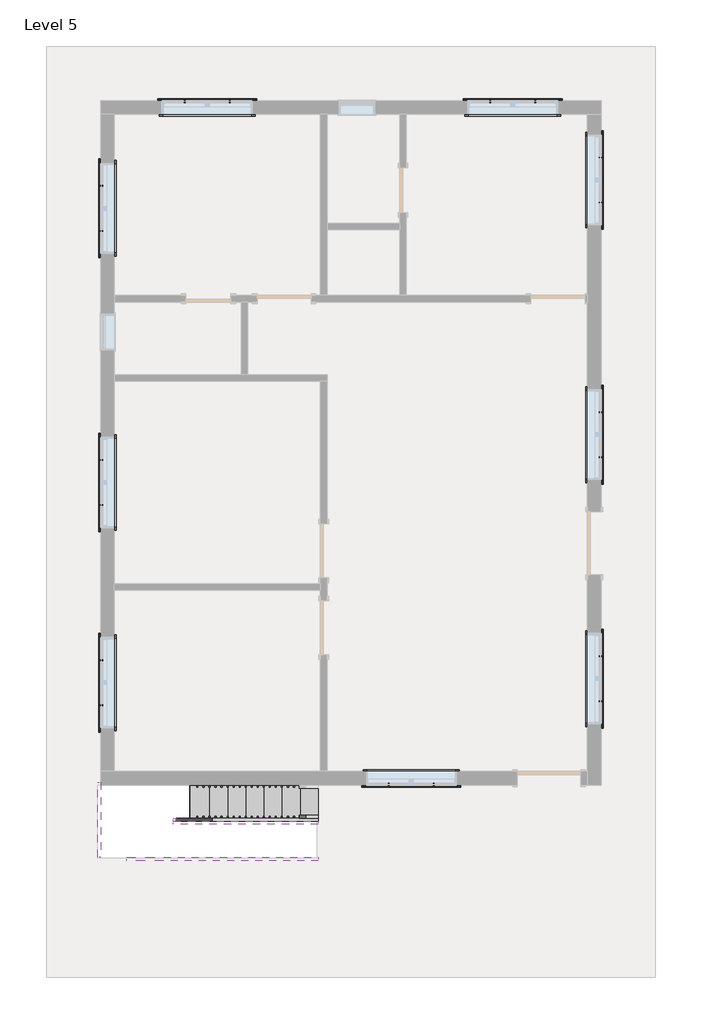
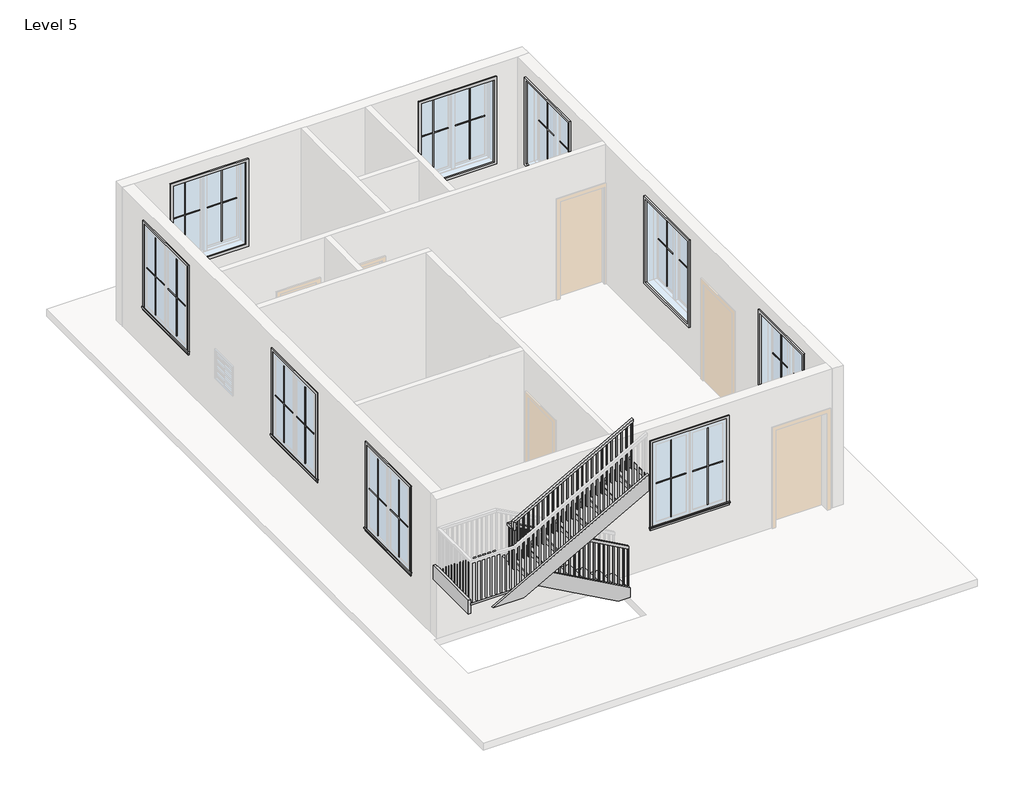
# One storey, part 3 of 3: 36 proxies, 6 members, 1 railing, 1 stair flight.
"""IFC4 building model written with IfcOpenShell, lengths in millimetres."""

from ifc_helpers import new_model, si_unit, frame, origin, place, context, project, spatial, polyline, outline, extrude, faceted_brep, transform, mapped, element, save
from components import muntin_pattern_2x2_muntin_pattern_2x2_f6a80940, muntin_pattern_2x2_muntin_pattern_2x2_09b00a1c, trim_window_exterior_flat_with_sill_698ed857, trim_window_interior_flat_picture_frame_92551a5e, stair_flight_d84c00c9

model = new_model("IFC4")

# Units and contexts
model_context = context("Model", 3, world=origin())
ifc_project = project(units=[si_unit("LENGTHUNIT", "METRE", prefix="MILLI")], contexts=[model_context])

# Site, building, storey
site = spatial("IfcSite", under=ifc_project)
building = spatial("IfcBuilding", under=site)
storey = spatial("IfcBuildingStorey", under=building, Name="Level 5", Elevation=9601.2)

# Proxies
placement = place(None, origin())
muntin_pattern_2x2_muntin_pattern_2x2_shape = muntin_pattern_2x2_muntin_pattern_2x2_f6a80940(model_context)
element("IfcBuildingElementProxy", 1, Name="Muntin Pattern_2x2 : Muntin Pattern_2x2", ObjectType="Muntin Pattern_2x2 : Muntin Pattern_2x2", at=placement, inside=storey, context=model_context, shape_type="MappedRepresentation", body=[
    mapped(muntin_pattern_2x2_muntin_pattern_2x2_shape, transform((-5453.9948569, -3961.7808037, 10585.45), x_axis=(0.0, 1.0, 0.0), y_axis=(-1.0, 0.0, 0.0), z_axis=(0.0, 0.0, 1.0))),
])
element("IfcBuildingElementProxy", 2, Name="Muntin Pattern_2x2 : Muntin Pattern_2x2", ObjectType="Muntin Pattern_2x2 : Muntin Pattern_2x2", at=placement, inside=storey, context=model_context, shape_type="MappedRepresentation", body=[
    mapped(muntin_pattern_2x2_muntin_pattern_2x2_shape, transform((-5453.9948569, -593.1058037, 10585.45), x_axis=(0.0, 1.0, 0.0), y_axis=(-1.0, 0.0, 0.0), z_axis=(0.0, 0.0, 1.0))),
])
element("IfcBuildingElementProxy", 3, Name="Muntin Pattern_2x2 : Muntin Pattern_2x2", ObjectType="Muntin Pattern_2x2 : Muntin Pattern_2x2", at=placement, inside=storey, context=model_context, shape_type="MappedRepresentation", body=[
    mapped(muntin_pattern_2x2_muntin_pattern_2x2_shape, transform((-5453.9948569, 4023.3441963, 10585.45), x_axis=(0.0, 1.0, 0.0), y_axis=(-1.0, 0.0, 0.0), z_axis=(0.0, 0.0, 1.0))),
])
element("IfcBuildingElementProxy", 4, Name="Muntin Pattern_2x2 : Muntin Pattern_2x2", ObjectType="Muntin Pattern_2x2 : Muntin Pattern_2x2", at=placement, inside=storey, context=model_context, shape_type="MappedRepresentation", body=[
    mapped(muntin_pattern_2x2_muntin_pattern_2x2_shape, transform((2947.0551431, 5258.4191963, 10585.45), x_axis=(0.0, -1.0, 0.0), y_axis=(1.0, 0.0, 0.0), z_axis=(0.0, 0.0, 1.0))),
])
element("IfcBuildingElementProxy", 5, Name="Muntin Pattern_2x2 : Muntin Pattern_2x2", ObjectType="Muntin Pattern_2x2 : Muntin Pattern_2x2", at=placement, inside=storey, context=model_context, shape_type="MappedRepresentation", body=[
    mapped(muntin_pattern_2x2_muntin_pattern_2x2_shape, transform((2947.0551431, 972.1691963, 10585.45), x_axis=(0.0, -1.0, 0.0), y_axis=(1.0, 0.0, 0.0), z_axis=(0.0, 0.0, 1.0))),
])
element("IfcBuildingElementProxy", 6, Name="Muntin Pattern_2x2 : Muntin Pattern_2x2", ObjectType="Muntin Pattern_2x2 : Muntin Pattern_2x2", at=placement, inside=storey, context=model_context, shape_type="MappedRepresentation", body=[
    mapped(muntin_pattern_2x2_muntin_pattern_2x2_shape, transform((2947.0551431, -3136.2808037, 10585.45), x_axis=(0.0, -1.0, 0.0), y_axis=(1.0, 0.0, 0.0), z_axis=(0.0, 0.0, 1.0))),
])
element("IfcBuildingElementProxy", 7, Name="Muntin Pattern_2x2 : Muntin Pattern_2x2", ObjectType="Muntin Pattern_2x2 : Muntin Pattern_2x2", at=placement, inside=storey, context=model_context, shape_type="MappedRepresentation", body=[
    mapped(muntin_pattern_2x2_muntin_pattern_2x2_shape, transform((141.9426431, -5296.8683037, 10585.45), x_axis=(-1.0, 0.0, 0.0), y_axis=(0.0, -1.0, 0.0), z_axis=(0.0, 0.0, 1.0))),
])
element("IfcBuildingElementProxy", 8, Name="Muntin Pattern_2x2 : Muntin Pattern_2x2", ObjectType="Muntin Pattern_2x2 : Muntin Pattern_2x2", at=placement, inside=storey, context=model_context, shape_type="MappedRepresentation", body=[
    mapped(muntin_pattern_2x2_muntin_pattern_2x2_shape, transform((1091.2676431, 6202.9816963, 10585.45), x_axis=(1.0, 0.0, 0.0), y_axis=(0.0, 1.0, 0.0), z_axis=(0.0, 0.0, 1.0))),
])
element("IfcBuildingElementProxy", 9, Name="Muntin Pattern_2x2 : Muntin Pattern_2x2", ObjectType="Muntin Pattern_2x2 : Muntin Pattern_2x2", at=placement, inside=storey, context=model_context, shape_type="MappedRepresentation", body=[
    mapped(muntin_pattern_2x2_muntin_pattern_2x2_shape, transform((-4052.2323569, 6202.9816963, 10585.45), x_axis=(1.0, 0.0, 0.0), y_axis=(0.0, 1.0, 0.0), z_axis=(0.0, 0.0, 1.0))),
])
muntin_pattern_2x2_muntin_pattern_2x2_2_shape = muntin_pattern_2x2_muntin_pattern_2x2_09b00a1c(model_context)
element("IfcBuildingElementProxy", 10, Name="Muntin Pattern_2x2 : Muntin Pattern_2x2", ObjectType="Muntin Pattern_2x2 : Muntin Pattern_2x2", at=placement, inside=storey, context=model_context, shape_type="MappedRepresentation", body=[
    mapped(muntin_pattern_2x2_muntin_pattern_2x2_2_shape, transform((-5453.9948569, -3202.9558037, 10585.45), x_axis=(0.0, -1.0, 0.0), y_axis=(1.0, 0.0, 0.0), z_axis=(0.0, 0.0, 1.0))),
])
element("IfcBuildingElementProxy", 11, Name="Muntin Pattern_2x2 : Muntin Pattern_2x2", ObjectType="Muntin Pattern_2x2 : Muntin Pattern_2x2", at=placement, inside=storey, context=model_context, shape_type="MappedRepresentation", body=[
    mapped(muntin_pattern_2x2_muntin_pattern_2x2_2_shape, transform((-5453.9948569, 165.7191963, 10585.45), x_axis=(0.0, -1.0, 0.0), y_axis=(1.0, 0.0, 0.0), z_axis=(0.0, 0.0, 1.0))),
])
element("IfcBuildingElementProxy", 12, Name="Muntin Pattern_2x2 : Muntin Pattern_2x2", ObjectType="Muntin Pattern_2x2 : Muntin Pattern_2x2", at=placement, inside=storey, context=model_context, shape_type="MappedRepresentation", body=[
    mapped(muntin_pattern_2x2_muntin_pattern_2x2_2_shape, transform((-5453.9948569, 4782.1691963, 10585.45), x_axis=(0.0, -1.0, 0.0), y_axis=(1.0, 0.0, 0.0), z_axis=(0.0, 0.0, 1.0))),
])
element("IfcBuildingElementProxy", 13, Name="Muntin Pattern_2x2 : Muntin Pattern_2x2", ObjectType="Muntin Pattern_2x2 : Muntin Pattern_2x2", at=placement, inside=storey, context=model_context, shape_type="MappedRepresentation", body=[
    mapped(muntin_pattern_2x2_muntin_pattern_2x2_2_shape, transform((2947.0551431, 4499.5941963, 10585.45), x_axis=(0.0, 1.0, 0.0), y_axis=(-1.0, 0.0, 0.0), z_axis=(0.0, 0.0, 1.0))),
])
element("IfcBuildingElementProxy", 14, Name="Muntin Pattern_2x2 : Muntin Pattern_2x2", ObjectType="Muntin Pattern_2x2 : Muntin Pattern_2x2", at=placement, inside=storey, context=model_context, shape_type="MappedRepresentation", body=[
    mapped(muntin_pattern_2x2_muntin_pattern_2x2_2_shape, transform((2947.0551431, 213.3441963, 10585.45), x_axis=(0.0, 1.0, 0.0), y_axis=(-1.0, 0.0, 0.0), z_axis=(0.0, 0.0, 1.0))),
])
element("IfcBuildingElementProxy", 15, Name="Muntin Pattern_2x2 : Muntin Pattern_2x2", ObjectType="Muntin Pattern_2x2 : Muntin Pattern_2x2", at=placement, inside=storey, context=model_context, shape_type="MappedRepresentation", body=[
    mapped(muntin_pattern_2x2_muntin_pattern_2x2_2_shape, transform((2947.0551431, -3895.1058037, 10585.45), x_axis=(0.0, 1.0, 0.0), y_axis=(-1.0, 0.0, 0.0), z_axis=(0.0, 0.0, 1.0))),
])
element("IfcBuildingElementProxy", 16, Name="Muntin Pattern_2x2 : Muntin Pattern_2x2", ObjectType="Muntin Pattern_2x2 : Muntin Pattern_2x2", at=placement, inside=storey, context=model_context, shape_type="MappedRepresentation", body=[
    mapped(muntin_pattern_2x2_muntin_pattern_2x2_2_shape, transform((-616.8823569, -5296.8683037, 10585.45), x_axis=(1.0, 0.0, 0.0), y_axis=(0.0, 1.0, 0.0), z_axis=(0.0, 0.0, 1.0))),
])
element("IfcBuildingElementProxy", 17, Name="Muntin Pattern_2x2 : Muntin Pattern_2x2", ObjectType="Muntin Pattern_2x2 : Muntin Pattern_2x2", at=placement, inside=storey, context=model_context, shape_type="MappedRepresentation", body=[
    mapped(muntin_pattern_2x2_muntin_pattern_2x2_2_shape, transform((1850.0926431, 6202.9816963, 10585.45), x_axis=(-1.0, 0.0, 0.0), y_axis=(0.0, -1.0, 0.0), z_axis=(0.0, 0.0, 1.0))),
])
element("IfcBuildingElementProxy", 18, Name="Muntin Pattern_2x2 : Muntin Pattern_2x2", ObjectType="Muntin Pattern_2x2 : Muntin Pattern_2x2", at=placement, inside=storey, context=model_context, shape_type="MappedRepresentation", body=[
    mapped(muntin_pattern_2x2_muntin_pattern_2x2_2_shape, transform((-3293.4073569, 6202.9816963, 10585.45), x_axis=(-1.0, 0.0, 0.0), y_axis=(0.0, -1.0, 0.0), z_axis=(0.0, 0.0, 1.0))),
])
trim_window_exterior_flat_with_sill_shape = trim_window_exterior_flat_with_sill_698ed857(model_context)
element("IfcBuildingElementProxy", 19, Name="Trim-Window-Exterior-Flat : with Sill", ObjectType="Trim-Window-Exterior-Flat : with Sill", at=placement, inside=storey, context=model_context, shape_type="MappedRepresentation", body=[
    mapped(trim_window_exterior_flat_with_sill_shape, transform((-5463.5198569, -3582.3683037, 12344.4), x_axis=(0.0, -1.0, 0.0), y_axis=(0.0, 0.0, 1.0), z_axis=(-1.0, 0.0, 0.0))),
])
element("IfcBuildingElementProxy", 20, Name="Trim-Window-Exterior-Flat : with Sill", ObjectType="Trim-Window-Exterior-Flat : with Sill", at=placement, inside=storey, context=model_context, shape_type="MappedRepresentation", body=[
    mapped(trim_window_exterior_flat_with_sill_shape, transform((-5463.5198569, -213.6933037, 12344.4), x_axis=(0.0, -1.0, 0.0), y_axis=(0.0, 0.0, 1.0), z_axis=(-1.0, 0.0, 0.0))),
])
element("IfcBuildingElementProxy", 21, Name="Trim-Window-Exterior-Flat : with Sill", ObjectType="Trim-Window-Exterior-Flat : with Sill", at=placement, inside=storey, context=model_context, shape_type="MappedRepresentation", body=[
    mapped(trim_window_exterior_flat_with_sill_shape, transform((-5463.5198569, 4402.7566963, 12344.4), x_axis=(0.0, -1.0, 0.0), y_axis=(0.0, 0.0, 1.0), z_axis=(-1.0, 0.0, 0.0))),
])
element("IfcBuildingElementProxy", 22, Name="Trim-Window-Exterior-Flat : with Sill", ObjectType="Trim-Window-Exterior-Flat : with Sill", at=placement, inside=storey, context=model_context, shape_type="MappedRepresentation", body=[
    mapped(trim_window_exterior_flat_with_sill_shape, transform((2956.5801431, 4879.0066963, 12344.4), x_axis=(0.0, 1.0, 0.0), y_axis=(0.0, 0.0, 1.0), z_axis=(1.0, 0.0, 0.0))),
])
element("IfcBuildingElementProxy", 23, Name="Trim-Window-Exterior-Flat : with Sill", ObjectType="Trim-Window-Exterior-Flat : with Sill", at=placement, inside=storey, context=model_context, shape_type="MappedRepresentation", body=[
    mapped(trim_window_exterior_flat_with_sill_shape, transform((2956.5801431, 592.7566963, 12344.4), x_axis=(0.0, 1.0, 0.0), y_axis=(0.0, 0.0, 1.0), z_axis=(1.0, 0.0, 0.0))),
])
element("IfcBuildingElementProxy", 24, Name="Trim-Window-Exterior-Flat : with Sill", ObjectType="Trim-Window-Exterior-Flat : with Sill", at=placement, inside=storey, context=model_context, shape_type="MappedRepresentation", body=[
    mapped(trim_window_exterior_flat_with_sill_shape, transform((2956.5801431, -3515.6933037, 12344.4), x_axis=(0.0, 1.0, 0.0), y_axis=(0.0, 0.0, 1.0), z_axis=(1.0, 0.0, 0.0))),
])
element("IfcBuildingElementProxy", 25, Name="Trim-Window-Exterior-Flat : with Sill", ObjectType="Trim-Window-Exterior-Flat : with Sill", at=placement, inside=storey, context=model_context, shape_type="MappedRepresentation", body=[
    mapped(trim_window_exterior_flat_with_sill_shape, transform((-237.4698569, -5306.3933037, 12344.4), x_axis=(1.0, 0.0, 0.0), y_axis=(0.0, 0.0, 1.0), z_axis=(0.0, -1.0, 0.0))),
])
element("IfcBuildingElementProxy", 26, Name="Trim-Window-Exterior-Flat : with Sill", ObjectType="Trim-Window-Exterior-Flat : with Sill", at=placement, inside=storey, context=model_context, shape_type="MappedRepresentation", body=[
    mapped(trim_window_exterior_flat_with_sill_shape, transform((1470.6801431, 6212.5066963, 12344.4), x_axis=(-1.0, 0.0, 0.0), y_axis=(0.0, 0.0, 1.0), z_axis=(0.0, 1.0, 0.0))),
])
element("IfcBuildingElementProxy", 27, Name="Trim-Window-Exterior-Flat : with Sill", ObjectType="Trim-Window-Exterior-Flat : with Sill", at=placement, inside=storey, context=model_context, shape_type="MappedRepresentation", body=[
    mapped(trim_window_exterior_flat_with_sill_shape, transform((-3672.8198569, 6212.5066963, 12344.4), x_axis=(-1.0, 0.0, 0.0), y_axis=(0.0, 0.0, 1.0), z_axis=(0.0, 1.0, 0.0))),
])
trim_window_interior_flat_picture_frame_shape = trim_window_interior_flat_picture_frame_92551a5e(model_context)
element("IfcBuildingElementProxy", 28, Name="Trim-Window-Interior-Flat : Picture Frame", ObjectType="Trim-Window-Interior-Flat : Picture Frame", at=placement, inside=storey, context=model_context, shape_type="MappedRepresentation", body=[
    mapped(trim_window_interior_flat_picture_frame_shape, transform((-5234.9198569, -3582.3683037, 12344.4), x_axis=(0.0, 1.0, 0.0), y_axis=(0.0, 0.0, 1.0), z_axis=(1.0, 0.0, 0.0))),
])
element("IfcBuildingElementProxy", 29, Name="Trim-Window-Interior-Flat : Picture Frame", ObjectType="Trim-Window-Interior-Flat : Picture Frame", at=placement, inside=storey, context=model_context, shape_type="MappedRepresentation", body=[
    mapped(trim_window_interior_flat_picture_frame_shape, transform((-5234.9198569, -213.6933037, 12344.4), x_axis=(0.0, 1.0, 0.0), y_axis=(0.0, 0.0, 1.0), z_axis=(1.0, 0.0, 0.0))),
])
element("IfcBuildingElementProxy", 30, Name="Trim-Window-Interior-Flat : Picture Frame", ObjectType="Trim-Window-Interior-Flat : Picture Frame", at=placement, inside=storey, context=model_context, shape_type="MappedRepresentation", body=[
    mapped(trim_window_interior_flat_picture_frame_shape, transform((-5234.9198569, 4402.7566963, 12344.4), x_axis=(0.0, 1.0, 0.0), y_axis=(0.0, 0.0, 1.0), z_axis=(1.0, 0.0, 0.0))),
])
element("IfcBuildingElementProxy", 31, Name="Trim-Window-Interior-Flat : Picture Frame", ObjectType="Trim-Window-Interior-Flat : Picture Frame", at=placement, inside=storey, context=model_context, shape_type="MappedRepresentation", body=[
    mapped(trim_window_interior_flat_picture_frame_shape, transform((2727.9801431, 4879.0066963, 12344.4), x_axis=(0.0, -1.0, 0.0), y_axis=(0.0, 0.0, 1.0), z_axis=(-1.0, 0.0, 0.0))),
])
element("IfcBuildingElementProxy", 32, Name="Trim-Window-Interior-Flat : Picture Frame", ObjectType="Trim-Window-Interior-Flat : Picture Frame", at=placement, inside=storey, context=model_context, shape_type="MappedRepresentation", body=[
    mapped(trim_window_interior_flat_picture_frame_shape, transform((2727.9801431, 592.7566963, 12344.4), x_axis=(0.0, -1.0, 0.0), y_axis=(0.0, 0.0, 1.0), z_axis=(-1.0, 0.0, 0.0))),
])
element("IfcBuildingElementProxy", 33, Name="Trim-Window-Interior-Flat : Picture Frame", ObjectType="Trim-Window-Interior-Flat : Picture Frame", at=placement, inside=storey, context=model_context, shape_type="MappedRepresentation", body=[
    mapped(trim_window_interior_flat_picture_frame_shape, transform((2727.9801431, -3515.6933037, 12344.4), x_axis=(0.0, -1.0, 0.0), y_axis=(0.0, 0.0, 1.0), z_axis=(-1.0, 0.0, 0.0))),
])
element("IfcBuildingElementProxy", 34, Name="Trim-Window-Interior-Flat : Picture Frame", ObjectType="Trim-Window-Interior-Flat : Picture Frame", at=placement, inside=storey, context=model_context, shape_type="MappedRepresentation", body=[
    mapped(trim_window_interior_flat_picture_frame_shape, transform((-237.4698569, -5077.7933037, 12344.4), x_axis=(-1.0, 0.0, 0.0), y_axis=(0.0, 0.0, 1.0), z_axis=(0.0, 1.0, 0.0))),
])
element("IfcBuildingElementProxy", 35, Name="Trim-Window-Interior-Flat : Picture Frame", ObjectType="Trim-Window-Interior-Flat : Picture Frame", at=placement, inside=storey, context=model_context, shape_type="MappedRepresentation", body=[
    mapped(trim_window_interior_flat_picture_frame_shape, transform((1470.6801431, 5983.9066963, 12344.4), x_axis=(1.0, 0.0, 0.0), y_axis=(0.0, 0.0, 1.0), z_axis=(0.0, -1.0, 0.0))),
])
element("IfcBuildingElementProxy", 36, Name="Trim-Window-Interior-Flat : Picture Frame", ObjectType="Trim-Window-Interior-Flat : Picture Frame", at=placement, inside=storey, context=model_context, shape_type="MappedRepresentation", body=[
    mapped(trim_window_interior_flat_picture_frame_shape, transform((-3672.8198569, 5983.9066963, 12344.4), x_axis=(1.0, 0.0, 0.0), y_axis=(0.0, 0.0, 1.0), z_axis=(0.0, -1.0, 0.0))),
])

# Members
element("IfcMember", 37, ObjectType="Stringer - 2\" Width", at=placement, inside=storey, context=model_context, shape_type="SweptSolid", body=[
    extrude(outline(polyline([(9601.2, -1805.9198569), (9808.7983948, -1805.9198569), (11135.2428392, -4193.5198569), (10786.5641651, -4193.5198569), (9601.2, -2059.8643597), (9601.2, -1805.9198569)])), frame((0.0, -5915.9933037, 0.0), z_axis=(0.0, 1.0, 0.0), x_axis=(0.0, 0.0, 1.0)), (0.0, 0.0, 1.0), 50.8),
])
element("IfcMember", 38, ObjectType="Stringer - 2\" Width", at=placement, inside=storey, context=model_context, shape_type="SweptSolid", body=[
    extrude(outline(polyline([(-4244.3198569, -5865.1933037), (-4193.5198569, -5865.1933037), (-4193.5198569, -5915.9933037), (-4244.3198569, -5915.9933037), (-4244.3198569, -5865.1933037)])), frame((0.0, 0.0, 10896.6), z_axis=(0.0, 0.0, 1.0), x_axis=(1.0, 0.0, 0.0)), (0.0, 0.0, 1.0), 304.8),
])
element("IfcMember", 39, ObjectType="Stringer - 2\" Width", at=placement, inside=storey, context=model_context, shape_type="SweptSolid", body=[
    extrude(outline(polyline([(11332.7983948, -4244.3198569), (10984.1197207, -4244.3198569), (12338.7863873, -1805.9198569), (12687.4650614, -1805.9198569), (11332.7983948, -4244.3198569)])), frame((0.0, -5966.7933037, 0.0), z_axis=(0.0, 1.0, 0.0), x_axis=(0.0, 0.0, 1.0)), (0.0, 0.0, 1.0), 50.8),
])
element("IfcMember", 40, ObjectType="Stringer - 2\" Width", at=placement, inside=storey, context=model_context, shape_type="SweptSolid", body=[
    extrude(outline(polyline([(9601.2, -1805.9198569), (9808.7983948, -1805.9198569), (11201.4, -4312.6027463), (11201.4, -4940.2243597), (9601.2, -2059.8643597), (9601.2, -1805.9198569)])), frame((0.0, -5306.3933037, 0.0), z_axis=(0.0, 1.0, 0.0), x_axis=(0.0, 0.0, 1.0)), (0.0, 0.0, 1.0), 50.8),
])
element("IfcMember", 41, ObjectType="Stringer - 2\" Width", at=placement, inside=storey, context=model_context, shape_type="SweptSolid", body=[
    extrude(outline(polyline([(-5514.3198569, -5255.5933037), (-5463.5198569, -5255.5933037), (-5463.5198569, -6525.5933037), (-5514.3198569, -6525.5933037), (-5514.3198569, -5255.5933037)])), frame((0.0, 0.0, 10896.6), z_axis=(0.0, 0.0, 1.0), x_axis=(1.0, 0.0, 0.0)), (0.0, 0.0, 1.0), 304.8),
])
element("IfcMember", 42, ObjectType="Stringer - 2\" Width", at=placement, inside=storey, context=model_context, shape_type="SweptSolid", body=[
    extrude(outline(polyline([(10896.6, -4401.8553541), (12338.7863873, -1805.9198569), (12687.4650614, -1805.9198569), (10896.6, -5029.4769675), (10896.6, -4401.8553541)])), frame((0.0, -6576.3933037, 0.0), z_axis=(0.0, 1.0, 0.0), x_axis=(0.0, 0.0, 1.0)), (0.0, 0.0, 1.0), 50.8),
])

# Railing
element("IfcRailing", 43, ObjectType="Handrail - Rectangular", at=placement, inside=storey, context=model_context, shape_type="SolidModel", body=[
    faceted_brep([(-1805.9198569, -5865.1933037, 10684.9333333), (-1805.9198569, -5865.1933037, 10626.820221), (-1805.9198569, -5814.3933037, 10626.820221), (-1805.9198569, -5814.3933037, 10684.9333333), (-4168.1198569, -5865.1933037, 11997.2666667), (-4218.9198569, -5865.1933037, 11967.3757765), (-4218.9198569, -5814.3933037, 11967.3757765), (-4168.1198569, -5814.3933037, 11997.2666667), (-4168.1198569, -5865.1933037, 12039.6), (-4218.9198569, -5865.1933037, 11988.8), (-4218.9198569, -5814.3933037, 11988.8), (-4168.1198569, -5814.3933037, 12039.6), (-4244.3198569, -5865.1933037, 12039.6), (-4244.3198569, -5865.1933037, 11988.8), (-4295.1198569, -5814.3933037, 11988.8), (-4295.1198569, -5814.3933037, 12039.6), (-4244.3198569, -5941.3933037, 12039.6), (-4244.3198569, -5941.3933037, 11988.8), (-4295.1198569, -5941.3933037, 11988.8), (-4295.1198569, -5941.3933037, 12039.6), (-4244.3198569, -5966.7933037, 12039.6), (-4295.1198569, -5966.7933037, 12039.6), (-4295.1198569, -6017.5933037, 11988.8), (-4244.3198569, -6017.5933037, 11988.8)], [[[0, 1, 2, 3]], [[1, 0, 4, 5]], [[2, 1, 5, 6]], [[3, 2, 6, 7]], [[0, 3, 7, 4]], [[5, 4, 8, 9]], [[6, 5, 9, 10]], [[7, 6, 10, 11]], [[4, 7, 11, 8]], [[9, 8, 12, 13]], [[10, 9, 13, 14]], [[11, 10, 14, 15]], [[8, 11, 15, 12]], [[13, 12, 16, 17]], [[14, 13, 17, 18]], [[15, 14, 18, 19]], [[12, 15, 19, 16]], [[20, 21, 22, 23]], [[17, 16, 20, 23]], [[18, 17, 23, 22]], [[19, 18, 22, 21]], [[16, 19, 21, 20]]]),
    faceted_brep([(-4244.3198569, -5966.7933037, 12039.6), (-4244.3198569, -6017.5933037, 11988.8), (-4295.1198569, -6017.5933037, 11988.8), (-4295.1198569, -5966.7933037, 12039.6), (-4244.3198569, -5966.7933037, 12150.820221), (-4295.1198569, -5966.7933037, 12180.7111111), (-4295.1198569, -6017.5933037, 12180.7111111), (-4244.3198569, -6017.5933037, 12150.820221)], [[[0, 1, 2, 3]], [[4, 5, 6, 7]], [[1, 0, 4, 7]], [[2, 1, 7, 6]], [[3, 2, 6, 5]], [[0, 3, 5, 4]]]),
    faceted_brep([(-4295.1198569, -5966.7933037, 12180.7111111), (-4244.3198569, -5966.7933037, 12150.820221), (-4244.3198569, -6017.5933037, 12150.820221), (-4295.1198569, -6017.5933037, 12180.7111111), (-1805.9198569, -5966.7933037, 13563.6), (-1805.9198569, -6017.5933037, 13563.6), (-1805.9198569, -6017.5933037, 13505.4868876), (-1805.9198569, -5966.7933037, 13505.4868876)], [[[0, 1, 2, 3]], [[4, 5, 6, 7]], [[1, 0, 4, 7]], [[2, 1, 7, 6]], [[3, 2, 6, 5]], [[0, 3, 5, 4]]]),
    extrude(outline(polyline([(13486.0841099, -1840.8448569), (12479.8666667, -1840.8448569), (12479.8666667, -1821.7948569), (13496.6674432, -1821.7948569), (13486.0841099, -1840.8448569)])), frame((0.0, -6001.7183037, 0.0), z_axis=(0.0, 1.0, 0.0), x_axis=(0.0, 0.0, 1.0)), (0.0, 0.0, 1.0), 19.05),
    extrude(outline(polyline([(13429.6396654, -1942.4448569), (12479.8666667, -1942.4448569), (12479.8666667, -1923.3948569), (13440.2229988, -1923.3948569), (13429.6396654, -1942.4448569)])), frame((0.0, -6001.7183037, 0.0), z_axis=(0.0, 1.0, 0.0), x_axis=(0.0, 0.0, 1.0)), (0.0, 0.0, 1.0), 19.05),
    extrude(outline(polyline([(13373.195221, -2044.0448569), (12479.8666667, -2044.0448569), (12479.8666667, -2024.9948569), (13383.7785543, -2024.9948569), (13373.195221, -2044.0448569)])), frame((0.0, -6001.7183037, 0.0), z_axis=(0.0, 1.0, 0.0), x_axis=(0.0, 0.0, 1.0)), (0.0, 0.0, 1.0), 19.05),
    extrude(outline(polyline([(13316.7507765, -2145.6448569), (12310.5333333, -2145.6448569), (12310.5333333, -2126.5948569), (13327.3341099, -2126.5948569), (13316.7507765, -2145.6448569)])), frame((0.0, -6001.7183037, 0.0), z_axis=(0.0, 1.0, 0.0), x_axis=(0.0, 0.0, 1.0)), (0.0, 0.0, 1.0), 19.05),
    extrude(outline(polyline([(13260.3063321, -2247.2448569), (12310.5333333, -2247.2448569), (12310.5333333, -2228.1948569), (13270.8896654, -2228.1948569), (13260.3063321, -2247.2448569)])), frame((0.0, -6001.7183037, 0.0), z_axis=(0.0, 1.0, 0.0), x_axis=(0.0, 0.0, 1.0)), (0.0, 0.0, 1.0), 19.05),
    extrude(outline(polyline([(13203.8618876, -2348.8448569), (12310.5333333, -2348.8448569), (12310.5333333, -2329.7948569), (13214.445221, -2329.7948569), (13203.8618876, -2348.8448569)])), frame((0.0, -6001.7183037, 0.0), z_axis=(0.0, 1.0, 0.0), x_axis=(0.0, 0.0, 1.0)), (0.0, 0.0, 1.0), 19.05),
    extrude(outline(polyline([(13147.4174432, -2450.4448569), (12141.2, -2450.4448569), (12141.2, -2431.3948569), (13158.0007765, -2431.3948569), (13147.4174432, -2450.4448569)])), frame((0.0, -6001.7183037, 0.0), z_axis=(0.0, 1.0, 0.0), x_axis=(0.0, 0.0, 1.0)), (0.0, 0.0, 1.0), 19.05),
    extrude(outline(polyline([(13090.9729988, -2552.0448569), (12141.2, -2552.0448569), (12141.2, -2532.9948569), (13101.5563321, -2532.9948569), (13090.9729988, -2552.0448569)])), frame((0.0, -6001.7183037, 0.0), z_axis=(0.0, 1.0, 0.0), x_axis=(0.0, 0.0, 1.0)), (0.0, 0.0, 1.0), 19.05),
    extrude(outline(polyline([(13034.5285543, -2653.6448569), (12141.2, -2653.6448569), (12141.2, -2634.5948569), (13045.1118876, -2634.5948569), (13034.5285543, -2653.6448569)])), frame((0.0, -6001.7183037, 0.0), z_axis=(0.0, 1.0, 0.0), x_axis=(0.0, 0.0, 1.0)), (0.0, 0.0, 1.0), 19.05),
    extrude(outline(polyline([(12978.0841099, -2755.2448569), (11971.8666667, -2755.2448569), (11971.8666667, -2736.1948569), (12988.6674432, -2736.1948569), (12978.0841099, -2755.2448569)])), frame((0.0, -6001.7183037, 0.0), z_axis=(0.0, 1.0, 0.0), x_axis=(0.0, 0.0, 1.0)), (0.0, 0.0, 1.0), 19.05),
    extrude(outline(polyline([(12921.6396654, -2856.8448569), (11971.8666667, -2856.8448569), (11971.8666667, -2837.7948569), (12932.2229988, -2837.7948569), (12921.6396654, -2856.8448569)])), frame((0.0, -6001.7183037, 0.0), z_axis=(0.0, 1.0, 0.0), x_axis=(0.0, 0.0, 1.0)), (0.0, 0.0, 1.0), 19.05),
    extrude(outline(polyline([(12865.195221, -2958.4448569), (11971.8666667, -2958.4448569), (11971.8666667, -2939.3948569), (12875.7785543, -2939.3948569), (12865.195221, -2958.4448569)])), frame((0.0, -6001.7183037, 0.0), z_axis=(0.0, 1.0, 0.0), x_axis=(0.0, 0.0, 1.0)), (0.0, 0.0, 1.0), 19.05),
    extrude(outline(polyline([(12808.7507765, -3060.0448569), (11802.5333333, -3060.0448569), (11802.5333333, -3040.9948569), (12819.3341099, -3040.9948569), (12808.7507765, -3060.0448569)])), frame((0.0, -6001.7183037, 0.0), z_axis=(0.0, 1.0, 0.0), x_axis=(0.0, 0.0, 1.0)), (0.0, 0.0, 1.0), 19.05),
    extrude(outline(polyline([(12752.3063321, -3161.6448569), (11802.5333333, -3161.6448569), (11802.5333333, -3142.5948569), (12762.8896654, -3142.5948569), (12752.3063321, -3161.6448569)])), frame((0.0, -6001.7183037, 0.0), z_axis=(0.0, 1.0, 0.0), x_axis=(0.0, 0.0, 1.0)), (0.0, 0.0, 1.0), 19.05),
    extrude(outline(polyline([(12695.8618876, -3263.2448569), (11802.5333333, -3263.2448569), (11802.5333333, -3244.1948569), (12706.445221, -3244.1948569), (12695.8618876, -3263.2448569)])), frame((0.0, -6001.7183037, 0.0), z_axis=(0.0, 1.0, 0.0), x_axis=(0.0, 0.0, 1.0)), (0.0, 0.0, 1.0), 19.05),
    extrude(outline(polyline([(12639.4174432, -3364.8448569), (11633.2, -3364.8448569), (11633.2, -3345.7948569), (12650.0007765, -3345.7948569), (12639.4174432, -3364.8448569)])), frame((0.0, -6001.7183037, 0.0), z_axis=(0.0, 1.0, 0.0), x_axis=(0.0, 0.0, 1.0)), (0.0, 0.0, 1.0), 19.05),
    extrude(outline(polyline([(12582.9729988, -3466.4448569), (11633.2, -3466.4448569), (11633.2, -3447.3948569), (12593.5563321, -3447.3948569), (12582.9729988, -3466.4448569)])), frame((0.0, -6001.7183037, 0.0), z_axis=(0.0, 1.0, 0.0), x_axis=(0.0, 0.0, 1.0)), (0.0, 0.0, 1.0), 19.05),
    extrude(outline(polyline([(12526.5285543, -3568.0448569), (11633.2, -3568.0448569), (11633.2, -3548.9948569), (12537.1118876, -3548.9948569), (12526.5285543, -3568.0448569)])), frame((0.0, -6001.7183037, 0.0), z_axis=(0.0, 1.0, 0.0), x_axis=(0.0, 0.0, 1.0)), (0.0, 0.0, 1.0), 19.05),
    extrude(outline(polyline([(12470.0841099, -3669.6448569), (11463.8666667, -3669.6448569), (11463.8666667, -3650.5948569), (12480.6674432, -3650.5948569), (12470.0841099, -3669.6448569)])), frame((0.0, -6001.7183037, 0.0), z_axis=(0.0, 1.0, 0.0), x_axis=(0.0, 0.0, 1.0)), (0.0, 0.0, 1.0), 19.05),
    extrude(outline(polyline([(12413.6396654, -3771.2448569), (11463.8666667, -3771.2448569), (11463.8666667, -3752.1948569), (12424.2229988, -3752.1948569), (12413.6396654, -3771.2448569)])), frame((0.0, -6001.7183037, 0.0), z_axis=(0.0, 1.0, 0.0), x_axis=(0.0, 0.0, 1.0)), (0.0, 0.0, 1.0), 19.05),
    extrude(outline(polyline([(12357.195221, -3872.8448569), (11463.8666667, -3872.8448569), (11463.8666667, -3853.7948569), (12367.7785543, -3853.7948569), (12357.195221, -3872.8448569)])), frame((0.0, -6001.7183037, 0.0), z_axis=(0.0, 1.0, 0.0), x_axis=(0.0, 0.0, 1.0)), (0.0, 0.0, 1.0), 19.05),
    extrude(outline(polyline([(12300.7507765, -3974.4448569), (11294.5333333, -3974.4448569), (11294.5333333, -3955.3948569), (12311.3341099, -3955.3948569), (12300.7507765, -3974.4448569)])), frame((0.0, -6001.7183037, 0.0), z_axis=(0.0, 1.0, 0.0), x_axis=(0.0, 0.0, 1.0)), (0.0, 0.0, 1.0), 19.05),
    extrude(outline(polyline([(12244.3063321, -4076.0448569), (11294.5333333, -4076.0448569), (11294.5333333, -4056.9948569), (12254.8896654, -4056.9948569), (12244.3063321, -4076.0448569)])), frame((0.0, -6001.7183037, 0.0), z_axis=(0.0, 1.0, 0.0), x_axis=(0.0, 0.0, 1.0)), (0.0, 0.0, 1.0), 19.05),
    extrude(outline(polyline([(12187.8618876, -4177.6448569), (11294.5333333, -4177.6448569), (11294.5333333, -4158.5948569), (12198.445221, -4158.5948569), (12187.8618876, -4177.6448569)])), frame((0.0, -6001.7183037, 0.0), z_axis=(0.0, 1.0, 0.0), x_axis=(0.0, 0.0, 1.0)), (0.0, 0.0, 1.0), 19.05),
    extrude(outline(polyline([(-4260.1948569, -5931.8683037), (-4260.1948569, -5950.9183037), (-4279.2448569, -5950.9183037), (-4279.2448569, -5931.8683037), (-4260.1948569, -5931.8683037)])), frame((0.0, 0.0, 11125.2), z_axis=(0.0, 0.0, 1.0), x_axis=(1.0, 0.0, 0.0)), (0.0, 0.0, 1.0), 863.6),
    extrude(outline(polyline([(-4234.7948569, -5849.3183037), (-4253.8448569, -5849.3183037), (-4253.8448569, -5830.2683037), (-4234.7948569, -5830.2683037), (-4234.7948569, -5849.3183037)])), frame((0.0, 0.0, 11125.2), z_axis=(0.0, 0.0, 1.0), x_axis=(1.0, 0.0, 0.0)), (0.0, 0.0, 1.0), 863.6),
    extrude(outline(polyline([(11930.3341099, -4152.2448569), (10955.8666667, -4152.2448569), (10955.8666667, -4133.1948569), (11919.7507765, -4133.1948569), (11930.3341099, -4152.2448569)])), frame((0.0, -5849.3183037, 0.0), z_axis=(0.0, 1.0, 0.0), x_axis=(0.0, 0.0, 1.0)), (0.0, 0.0, 1.0), 19.05),
    extrude(outline(polyline([(11873.8896654, -4050.6448569), (10955.8666667, -4050.6448569), (10955.8666667, -4031.5948569), (11863.3063321, -4031.5948569), (11873.8896654, -4050.6448569)])), frame((0.0, -5849.3183037, 0.0), z_axis=(0.0, 1.0, 0.0), x_axis=(0.0, 0.0, 1.0)), (0.0, 0.0, 1.0), 19.05),
    extrude(outline(polyline([(11817.445221, -3949.0448569), (10955.8666667, -3949.0448569), (10955.8666667, -3929.9948569), (11806.8618876, -3929.9948569), (11817.445221, -3949.0448569)])), frame((0.0, -5849.3183037, 0.0), z_axis=(0.0, 1.0, 0.0), x_axis=(0.0, 0.0, 1.0)), (0.0, 0.0, 1.0), 19.05),
    extrude(outline(polyline([(11761.0007765, -3847.4448569), (10786.5333333, -3847.4448569), (10786.5333333, -3828.3948569), (11750.4174432, -3828.3948569), (11761.0007765, -3847.4448569)])), frame((0.0, -5849.3183037, 0.0), z_axis=(0.0, 1.0, 0.0), x_axis=(0.0, 0.0, 1.0)), (0.0, 0.0, 1.0), 19.05),
    extrude(outline(polyline([(11704.5563321, -3745.8448569), (10786.5333333, -3745.8448569), (10786.5333333, -3726.7948569), (11693.9729988, -3726.7948569), (11704.5563321, -3745.8448569)])), frame((0.0, -5849.3183037, 0.0), z_axis=(0.0, 1.0, 0.0), x_axis=(0.0, 0.0, 1.0)), (0.0, 0.0, 1.0), 19.05),
    extrude(outline(polyline([(11648.1118876, -3644.2448569), (10786.5333333, -3644.2448569), (10786.5333333, -3625.1948569), (11637.5285543, -3625.1948569), (11648.1118876, -3644.2448569)])), frame((0.0, -5849.3183037, 0.0), z_axis=(0.0, 1.0, 0.0), x_axis=(0.0, 0.0, 1.0)), (0.0, 0.0, 1.0), 19.05),
    extrude(outline(polyline([(11591.6674432, -3542.6448569), (10617.2, -3542.6448569), (10617.2, -3523.5948569), (11581.0841099, -3523.5948569), (11591.6674432, -3542.6448569)])), frame((0.0, -5849.3183037, 0.0), z_axis=(0.0, 1.0, 0.0), x_axis=(0.0, 0.0, 1.0)), (0.0, 0.0, 1.0), 19.05),
    extrude(outline(polyline([(11535.2229988, -3441.0448569), (10617.2, -3441.0448569), (10617.2, -3421.9948569), (11524.6396654, -3421.9948569), (11535.2229988, -3441.0448569)])), frame((0.0, -5849.3183037, 0.0), z_axis=(0.0, 1.0, 0.0), x_axis=(0.0, 0.0, 1.0)), (0.0, 0.0, 1.0), 19.05),
    extrude(outline(polyline([(11478.7785543, -3339.4448569), (10617.2, -3339.4448569), (10617.2, -3320.3948569), (11468.195221, -3320.3948569), (11478.7785543, -3339.4448569)])), frame((0.0, -5849.3183037, 0.0), z_axis=(0.0, 1.0, 0.0), x_axis=(0.0, 0.0, 1.0)), (0.0, 0.0, 1.0), 19.05),
    extrude(outline(polyline([(11422.3341099, -3237.8448569), (10447.8666667, -3237.8448569), (10447.8666667, -3218.7948569), (11411.7507765, -3218.7948569), (11422.3341099, -3237.8448569)])), frame((0.0, -5849.3183037, 0.0), z_axis=(0.0, 1.0, 0.0), x_axis=(0.0, 0.0, 1.0)), (0.0, 0.0, 1.0), 19.05),
    extrude(outline(polyline([(11365.8896654, -3136.2448569), (10447.8666667, -3136.2448569), (10447.8666667, -3117.1948569), (11355.3063321, -3117.1948569), (11365.8896654, -3136.2448569)])), frame((0.0, -5849.3183037, 0.0), z_axis=(0.0, 1.0, 0.0), x_axis=(0.0, 0.0, 1.0)), (0.0, 0.0, 1.0), 19.05),
    extrude(outline(polyline([(11309.445221, -3034.6448569), (10447.8666667, -3034.6448569), (10447.8666667, -3015.5948569), (11298.8618876, -3015.5948569), (11309.445221, -3034.6448569)])), frame((0.0, -5849.3183037, 0.0), z_axis=(0.0, 1.0, 0.0), x_axis=(0.0, 0.0, 1.0)), (0.0, 0.0, 1.0), 19.05),
    extrude(outline(polyline([(11253.0007765, -2933.0448569), (10278.5333333, -2933.0448569), (10278.5333333, -2913.9948569), (11242.4174432, -2913.9948569), (11253.0007765, -2933.0448569)])), frame((0.0, -5849.3183037, 0.0), z_axis=(0.0, 1.0, 0.0), x_axis=(0.0, 0.0, 1.0)), (0.0, 0.0, 1.0), 19.05),
    extrude(outline(polyline([(11196.5563321, -2831.4448569), (10278.5333333, -2831.4448569), (10278.5333333, -2812.3948569), (11185.9729988, -2812.3948569), (11196.5563321, -2831.4448569)])), frame((0.0, -5849.3183037, 0.0), z_axis=(0.0, 1.0, 0.0), x_axis=(0.0, 0.0, 1.0)), (0.0, 0.0, 1.0), 19.05),
    extrude(outline(polyline([(11140.1118876, -2729.8448569), (10278.5333333, -2729.8448569), (10278.5333333, -2710.7948569), (11129.5285543, -2710.7948569), (11140.1118876, -2729.8448569)])), frame((0.0, -5849.3183037, 0.0), z_axis=(0.0, 1.0, 0.0), x_axis=(0.0, 0.0, 1.0)), (0.0, 0.0, 1.0), 19.05),
    extrude(outline(polyline([(11083.6674432, -2628.2448569), (10109.2, -2628.2448569), (10109.2, -2609.1948569), (11073.0841099, -2609.1948569), (11083.6674432, -2628.2448569)])), frame((0.0, -5849.3183037, 0.0), z_axis=(0.0, 1.0, 0.0), x_axis=(0.0, 0.0, 1.0)), (0.0, 0.0, 1.0), 19.05),
    extrude(outline(polyline([(11027.2229988, -2526.6448569), (10109.2, -2526.6448569), (10109.2, -2507.5948569), (11016.6396654, -2507.5948569), (11027.2229988, -2526.6448569)])), frame((0.0, -5849.3183037, 0.0), z_axis=(0.0, 1.0, 0.0), x_axis=(0.0, 0.0, 1.0)), (0.0, 0.0, 1.0), 19.05),
    extrude(outline(polyline([(10970.7785543, -2425.0448569), (10109.2, -2425.0448569), (10109.2, -2405.9948569), (10960.195221, -2405.9948569), (10970.7785543, -2425.0448569)])), frame((0.0, -5849.3183037, 0.0), z_axis=(0.0, 1.0, 0.0), x_axis=(0.0, 0.0, 1.0)), (0.0, 0.0, 1.0), 19.05),
    extrude(outline(polyline([(10914.3341099, -2323.4448569), (9939.8666667, -2323.4448569), (9939.8666667, -2304.3948569), (10903.7507765, -2304.3948569), (10914.3341099, -2323.4448569)])), frame((0.0, -5849.3183037, 0.0), z_axis=(0.0, 1.0, 0.0), x_axis=(0.0, 0.0, 1.0)), (0.0, 0.0, 1.0), 19.05),
    extrude(outline(polyline([(10857.8896654, -2221.8448569), (9939.8666667, -2221.8448569), (9939.8666667, -2202.7948569), (10847.3063321, -2202.7948569), (10857.8896654, -2221.8448569)])), frame((0.0, -5849.3183037, 0.0), z_axis=(0.0, 1.0, 0.0), x_axis=(0.0, 0.0, 1.0)), (0.0, 0.0, 1.0), 19.05),
    extrude(outline(polyline([(10801.445221, -2120.2448569), (9939.8666667, -2120.2448569), (9939.8666667, -2101.1948569), (10790.8618876, -2101.1948569), (10801.445221, -2120.2448569)])), frame((0.0, -5849.3183037, 0.0), z_axis=(0.0, 1.0, 0.0), x_axis=(0.0, 0.0, 1.0)), (0.0, 0.0, 1.0), 19.05),
    extrude(outline(polyline([(10745.0007765, -2018.6448569), (9770.5333333, -2018.6448569), (9770.5333333, -1999.5948569), (10734.4174432, -1999.5948569), (10745.0007765, -2018.6448569)])), frame((0.0, -5849.3183037, 0.0), z_axis=(0.0, 1.0, 0.0), x_axis=(0.0, 0.0, 1.0)), (0.0, 0.0, 1.0), 19.05),
    extrude(outline(polyline([(10688.5563321, -1917.0448569), (9770.5333333, -1917.0448569), (9770.5333333, -1897.9948569), (10677.9729988, -1897.9948569), (10688.5563321, -1917.0448569)])), frame((0.0, -5849.3183037, 0.0), z_axis=(0.0, 1.0, 0.0), x_axis=(0.0, 0.0, 1.0)), (0.0, 0.0, 1.0), 19.05),
    extrude(outline(polyline([(-4260.1948569, -5982.6683037), (-4260.1948569, -6001.7183037), (-4279.2448569, -6001.7183037), (-4279.2448569, -5982.6683037), (-4260.1948569, -5982.6683037)])), frame((0.0, 0.0, 11125.2), z_axis=(0.0, 0.0, 1.0), x_axis=(1.0, 0.0, 0.0)), (0.0, 0.0, 1.0), 863.6),
    extrude(outline(polyline([(-4260.1948569, -5849.3183037), (-4279.2448569, -5849.3183037), (-4279.2448569, -5830.2683037), (-4260.1948569, -5830.2683037), (-4260.1948569, -5849.3183037)])), frame((0.0, 0.0, 11125.2), z_axis=(0.0, 0.0, 1.0), x_axis=(1.0, 0.0, 0.0)), (0.0, 0.0, 1.0), 863.6),
    extrude(outline(polyline([(13494.9035543, -1824.9698569), (12479.8666667, -1824.9698569), (12479.8666667, -1805.9198569), (13505.4868876, -1805.9198569), (13494.9035543, -1824.9698569)])), frame((0.0, -6001.7183037, 0.0), z_axis=(0.0, 1.0, 0.0), x_axis=(0.0, 0.0, 1.0)), (0.0, 0.0, 1.0), 19.05),
    extrude(outline(polyline([(10637.4035543, -1824.9698569), (9770.5333333, -1824.9698569), (9770.5333333, -1805.9198569), (10626.820221, -1805.9198569), (10637.4035543, -1824.9698569)])), frame((0.0, -5849.3183037, 0.0), z_axis=(0.0, 1.0, 0.0), x_axis=(0.0, 0.0, 1.0)), (0.0, 0.0, 1.0), 19.05),
])

# Stair flight
stair_flight_shape = stair_flight_d84c00c9(model_context)
element("IfcStairFlight", 44, ObjectType="2\" Tread 1\" Nosing 1/4\" Riser", at=placement, inside=storey, context=model_context, shape_type="MappedRepresentation", body=[
    mapped(stair_flight_shape, transform((0.0, 0.0, 0.0), x_axis=(1.0, 0.0, 0.0), y_axis=(0.0, 1.0, 0.0), z_axis=(0.0, 0.0, 1.0))),
])

save(model, "model.ifc")

# Revit data of these elements
# Type "Muntin Pattern_2x2 : Muntin Pattern_2x2"
#   Width [instance default] = 4' - 0"
#   Thickness = 0' - 0 1/2"
#   Height [instance default] = 4' - 0"
#   Distance = 0' - 0 3/4"
#   Interior Material [instance default] = none
#   Exterior Material [instance default] = none
#   Default Elevation = 0
# Type "Trim-Window-Exterior-Flat : with Sill"
#   Trim Width = 0' - 2 1/4"
#   Trim Thickness_Picture Frame = 0' - 1 1/4"
#   Trim Thickness_with Sill = 0' - 0 3/4"
#   Sill Thickness = 0' - 1 1/4"
#   Opening Width [instance default] = 2' - 0"
#   Opening Height [instance default] = 3' - 0"
#   Default Elevation = 4' - 0"
#   Sill = yes
#   Picture Frame = no
#   Trim Material [instance default] = none
# Type "Trim-Window-Interior-Flat : Picture Frame"
#   Trim Thickness_Picture Frame = 0' - 1 1/4"
#   Trim Width = 0' - 2 1/4"
#   Trim Thickness_with Sill = 0' - 0 3/4"
#   Sill Thickness = 0' - 1 1/4"
#   Opening Width [instance default] = 2' - 0"
#   Opening Height [instance default] = 3' - 0"
#   Default Elevation = 4' - 0"
#   Sill = no
#   Picture Frame = yes
#   Trim Material [instance default] = none
# Type "Handrail - Rectangular"
#   Assembly Code = "C2010400"
#   built-in parameter 1008612 = 0.0416667 (stored number, unit not read)
#   built-in parameter 1008611 = 0.0416667 (stored number, unit not read)
#   built-in parameter 1008609 = 0.333333 (stored number, unit not read)
#   built-in parameter 1008604 = 0.166667 (stored number, unit not read)
#   built-in parameter 1008603 = 0.166667 (stored number, unit not read)
#   Railing Height = 3' - 0"
#   built-in parameter 1008630 = 2
#   built-in parameter 1008610 = 2
#   built-in parameter 1008618 = Baluster - Square : 3/4"
# Elements 1, 2, 3, 4, 5, 6, 7, 8, 9, 10, 11, 12, 13, 14, 15, 16, 17, 18 (IfcBuildingElementProxy, "Muntin Pattern_2x2 : Muntin Pattern_2x2")
#   Width = 2' - 0 5/8"
#   Height = 5' - 6 1/2"
#   Interior Material = Wood - Stained
#   Exterior Material = Clad - White
#   Phase Created = New Construction
#   Materials on its faces: "Clad - White", "Wood - Stained"
# Elements 19, 20, 21, 22, 23, 24, 25, 26, 27 (IfcBuildingElementProxy, "Trim-Window-Exterior-Flat : with Sill")
#   Opening Width = 5' - 0"
#   Opening Height = 6' - 0"
#   Trim Material = Clad - White
#   Phase Created = New Construction
#   Materials on its faces: "Clad - White"
# Elements 28, 29, 30, 31, 32, 33, 34, 35, 36 (IfcBuildingElementProxy, "Trim-Window-Interior-Flat : Picture Frame")
#   Opening Width = 5' - 0"
#   Opening Height = 6' - 0"
#   Trim Material = Wood - Stained
#   Phase Created = New Construction
#   Materials on its faces: "Wood - Stained"
# Elements 37, 38, 39, 40, 41, 42 (IfcMember, "Stringer - 2\" Width")
#   Phase Created = New Construction
# Element 43 (IfcRailing, "Handrail - Rectangular")
#   Phase Created = New Construction
# Element 44 (IfcStairFlight, "2\" Tread 1\" Nosing 1/4\" Riser")
#   Phase Created = New Construction
# Materials
#   "Clad - White": class "Wood", colour RGB 242 242 238, transparency 0, Cost = 0
#   "Wood - Stained": class "Wood", colour RGB 224 178 126, transparency 0, Cost = 0
